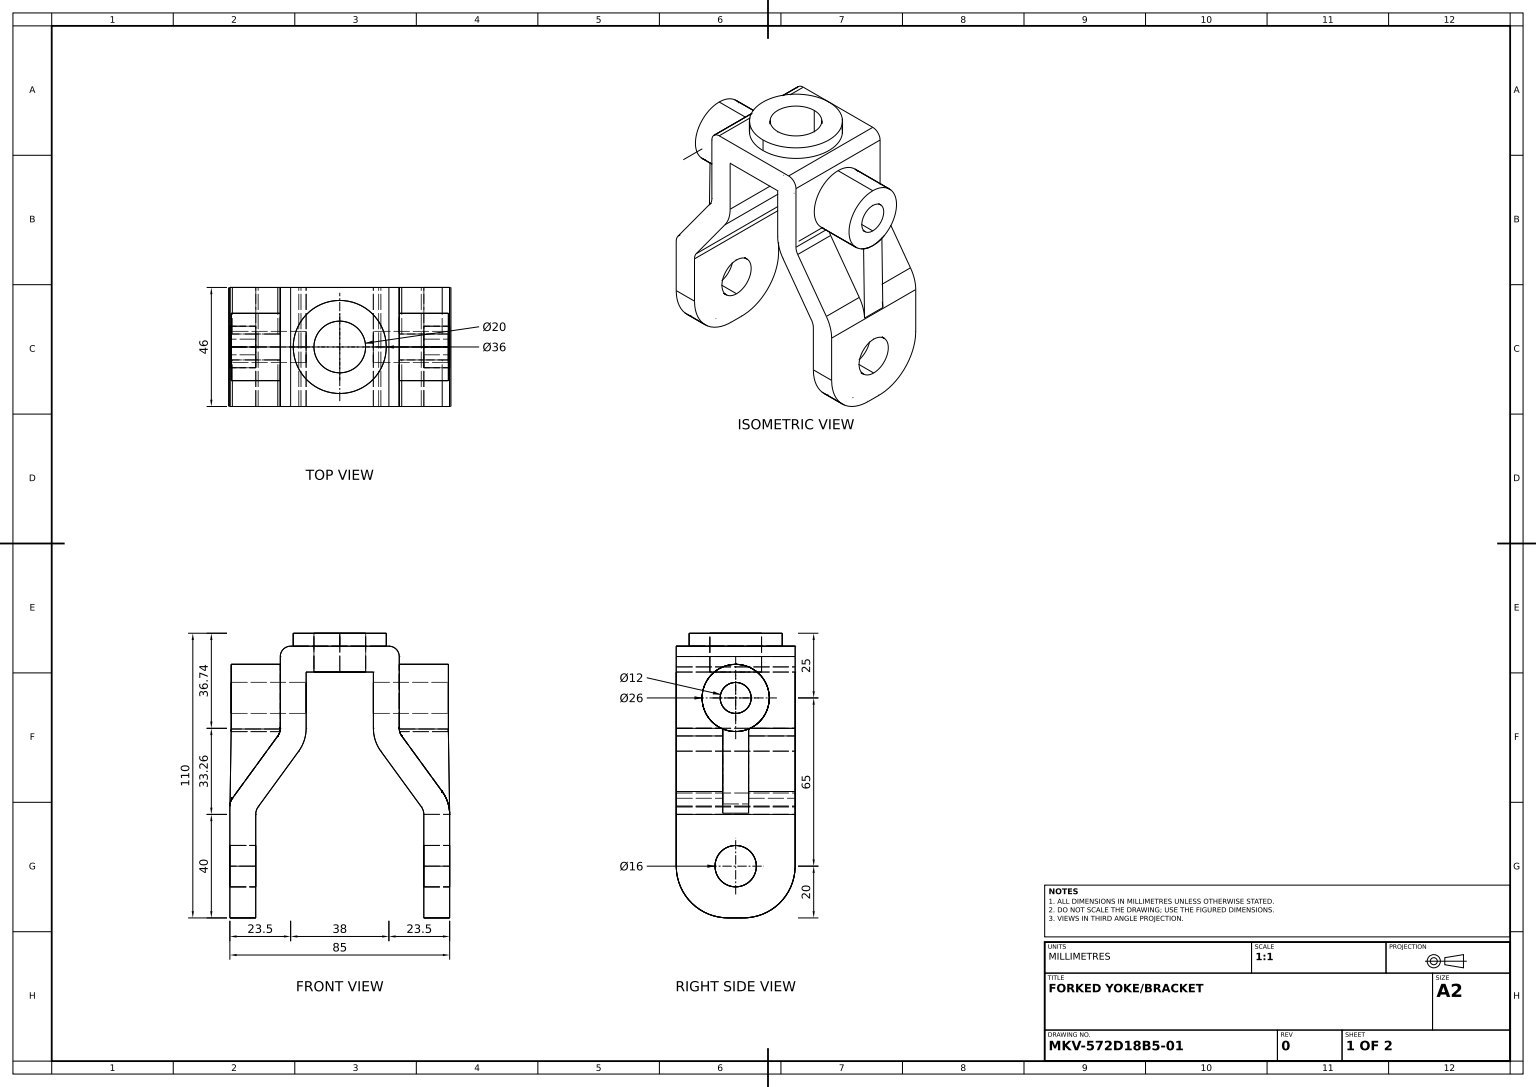
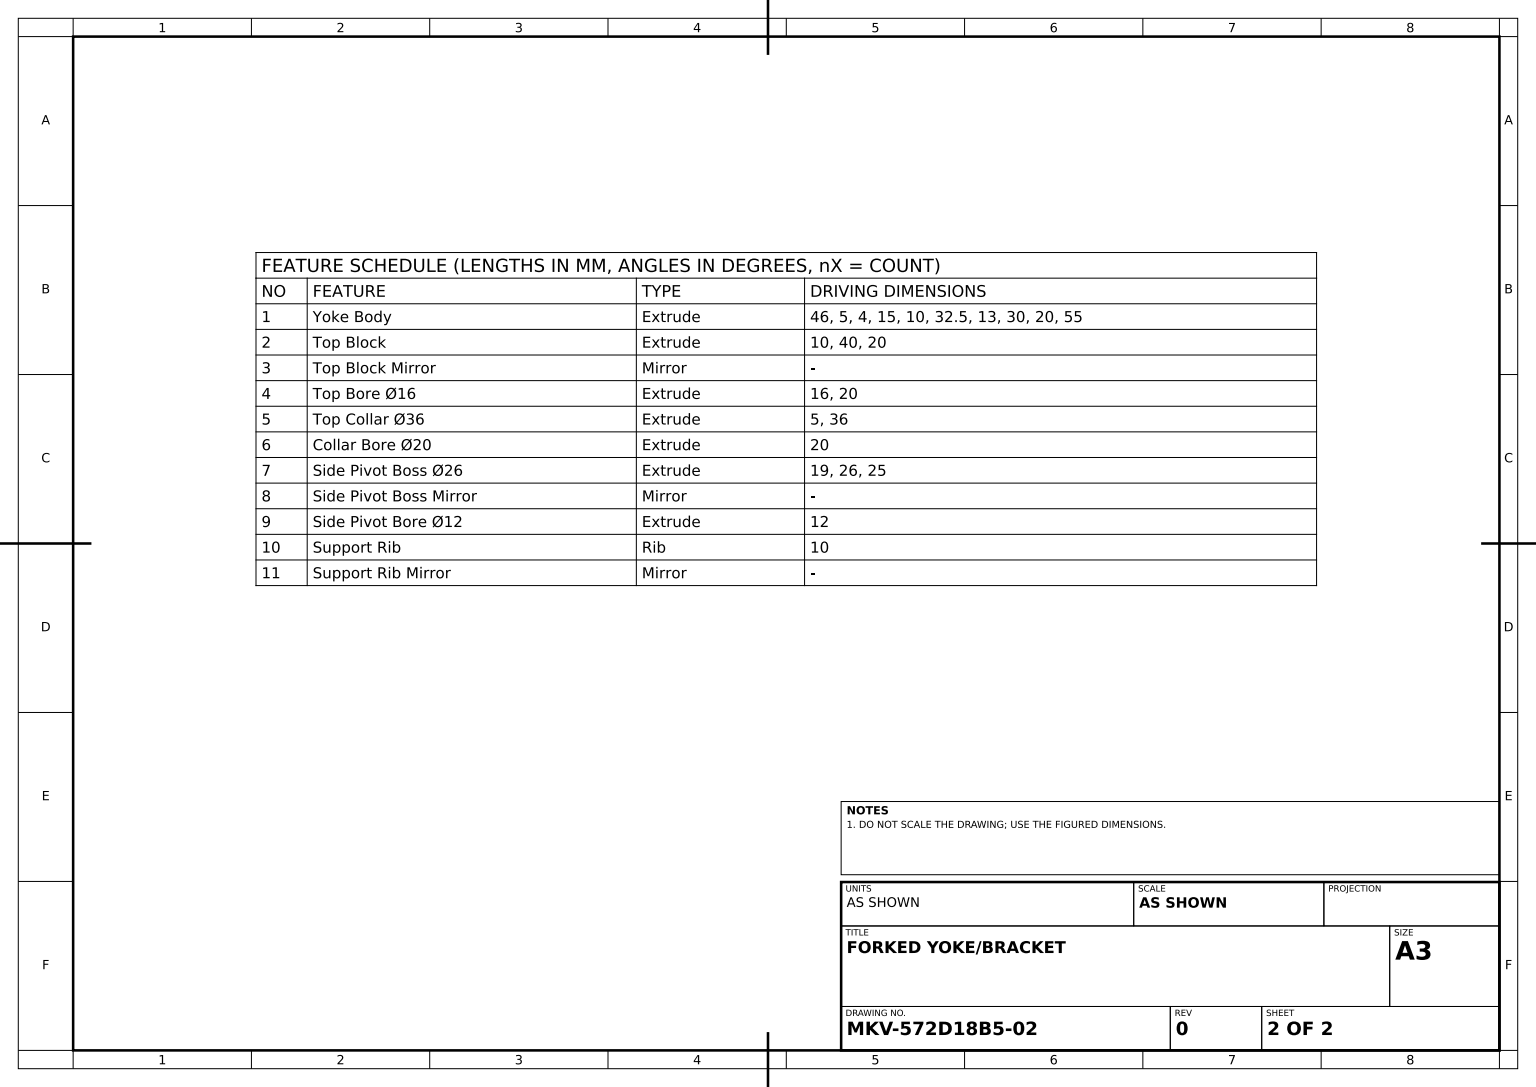
SolidWorks part; units mm, degrees
material "Plain Carbon Steel"
ref_plane "Front Plane" through (0, 0, 0) normal (0, 0, 1) x (1, 0, 0)
ref_plane "Top Plane" through (0, 0, 0) normal (0, 1, 0) x (1, 0, 0)
ref_plane "Right Plane" through (0, 0, 0) normal (1, 0, 0) x (0, 0, -1)
sketch "Yoke Profile Sketch" plane through (0, 0, 0) normal (0, 0, 1) x (1, 0, 0)
  line L8 (19, 10) -> (-19, 10)
  line L9 (0, 0) -> (0, 46.9956) construction
  line L10 (-32.5, -71.7411) -> (-42.5, -71.7411)
  line L11 (-23, -21.7411) -> (-23, 6)
  line L12 (-41.5399, -48.7952) -> (-23.9601, -24.6871)
  line L13 (-42.5, -71.7411) -> (-42.5, -51.7411)
  line L14 (-32.5, -55) -> (-32.5, -71.7411)
  line L17 (-31.5399, -52.054) -> (-15.8802, -30.5791)
  line L18 (-13, -21.7411) -> (-13, 0)
  line L21 (13, 0) -> (-13, 0)
  line L22 (23, -21.7411) -> (23, 6)
  line L23 (13, -21.7411) -> (13, 0)
  line L24 (32.5, -71.7411) -> (42.5, -71.7411)
  line L25 (32.5, -55) -> (32.5, -71.7411)
  line L26 (42.5, -71.7411) -> (42.5, -55)
  line L27 (31.5399, -52.054) -> (15.8802, -30.5791)
  line L28 (39.6198, -46.162) -> (23.9601, -24.6871)
  arc A0 (-23, -21.7411) -> (-23.9601, -24.6871) centre (-28, -21.7411) cw
  arc A4 (-23, 6) -> (-19, 10) centre (-19, 6) cw
  arc A5 (23, 6) -> (19, 10) centre (19, 6) ccw
  arc A6 (-15.8802, -30.5791) -> (-13, -21.7411) centre (-28, -21.7411) ccw
  arc A8 (15.8802, -30.5791) -> (13, -21.7411) centre (28, -21.7411) cw
  arc A9 (23, -21.7411) -> (23.9601, -24.6871) centre (28, -21.7411) ccw
  arc A10 (-32.5, -55) -> (-31.5399, -52.054) centre (-27.5, -55) cw
  arc A11 (-41.5399, -48.7952) -> (-42.5, -51.7411) centre (-37.5, -51.7411) ccw
  arc A12 (32.5, -55) -> (31.5399, -52.054) centre (27.5, -55) ccw
  arc A13 (42.5, -55) -> (39.6198, -46.162) centre (27.5, -55) ccw
  point P16 (0, 10)
  point P23 (-23, -23.3706)
  point P26 (23, -23.3706)
  point P35 (-23, 10)
  point P38 (23, 10)
  point P40 (-32.5, -53.3706)
  point P43 (-42.5, -50.1117)
  point P46 (32.5, -53.3706)
  point P49 (42.5, -50.1117)
  dimension "D3" = 5
  dimension "D4" = 15
  dimension "D5" = 4
  dimension "D7" = 5
  dimension "D8" = 5
  dimension "D9" = 15
  dimension "D2" = 20
  dimension "D6" = 10
  dimension "D10" = 32.5
  dimension "D11" = 10
  dimension "D12" = 13
  dimension "D13" = 55
  dimension "D14" = 30
extrude "Yoke Body" add sketch "Yoke Profile Sketch" along normal mid plane 46
sketch "Top Block Sketch" plane through (42.5, 0, 0) normal (1, 0, 0) x (0, 0, -1)
  line L0 (-3, -95) -> (3, -95)
  line L1 (-23, -71.7411) -> (23, -71.7411)
  line L2 (-23, -71.7411) -> (-23, -75)
  line L3 (23, -71.7411) -> (23, -75)
  line L4 (-23, -55) -> (23, -55) construction
  line L5 (0, -69.6852) -> (0, -115.0343) construction
  arc A0 (-23, -75) -> (-3, -95) centre (-3, -75) ccw
  arc A1 (23, -75) -> (3, -95) centre (3, -75) cw
  dimension "D2" = 20
  dimension "D1" = 40
extrude "Top Block" add sketch "Top Block Sketch" against normal blind 10 contours A0 L0 A1 L3 L1 L2
mirror "Top Block Mirror" about plane through (0, 0, 0) normal (1, 0, 0) of "Top Block"
sketch "Top Bore Sketch" plane through (42.5, 0, 0) normal (1, 0, 0) x (0, 0, -1)
  line L0 (-3, -95) -> (3, -95) construction
  circle A0 centre (0, -75) radius 8
  dimension "D1" = 16
  dimension "D2" = 20
extrude "Top Bore Ø16" cut sketch "Top Bore Sketch" against normal through all
sketch "Top Collar Sketch" plane through (0, 10, 0) normal (0, 1, 0) x (1, 0, 0)
  circle A0 centre (0, 0) radius 18
  dimension "D1" = 36
extrude "Top Collar Ø36" add sketch "Top Collar Sketch" along normal blind 5
sketch "Collar Bore Sketch" plane through (0, 15, 0) normal (0, 1, 0) x (1, 0, 0)
  circle A0 centre (0, 0) radius 10
  dimension "D1" = 20
extrude "Collar Bore Ø20" cut sketch "Collar Bore Sketch" against normal up to next
sketch "Side Pivot Boss Sketch" plane through (23, 0, 0) normal (1, 0, 0) x (0, 0, -1)
  line L0 (18, 15) -> (-18, 15) construction
  circle A0 centre (0, -10) radius 13
  dimension "D1" = 26
  dimension "D2" = 25
extrude "Side Pivot Boss Ø26" add sketch "Side Pivot Boss Sketch" along normal blind 19
mirror "Side Pivot Boss Mirror" about plane through (0, 0, 0) normal (1, 0, 0) of "Side Pivot Boss Ø26"
sketch "Side Pivot Bore Sketch" plane through (42, 0, 0) normal (1, 0, 0) x (0, 0, -1)
  circle A0 centre (0, -10) radius 6
  circle A1 centre (0, -10) radius 13 construction
  dimension "D1" = 12
extrude "Side Pivot Bore Ø12" cut sketch "Side Pivot Bore Sketch" against normal through all
sketch "Support Rib Sketch" plane through (0, 0, 0) normal (0, 0, 1) x (1, 0, 0)
  line L0 (42, -23) -> (42.5, -55)
rib "Support Rib" sketch "Support Rib Sketch" sketch "Support Rib Sketch" thickness 10 extrusion direction parallel to sketch draft on no parameters "D1"=10
mirror "Support Rib Mirror" about plane through (0, 0, 0) normal (1, 0, 0) of "Support Rib"
